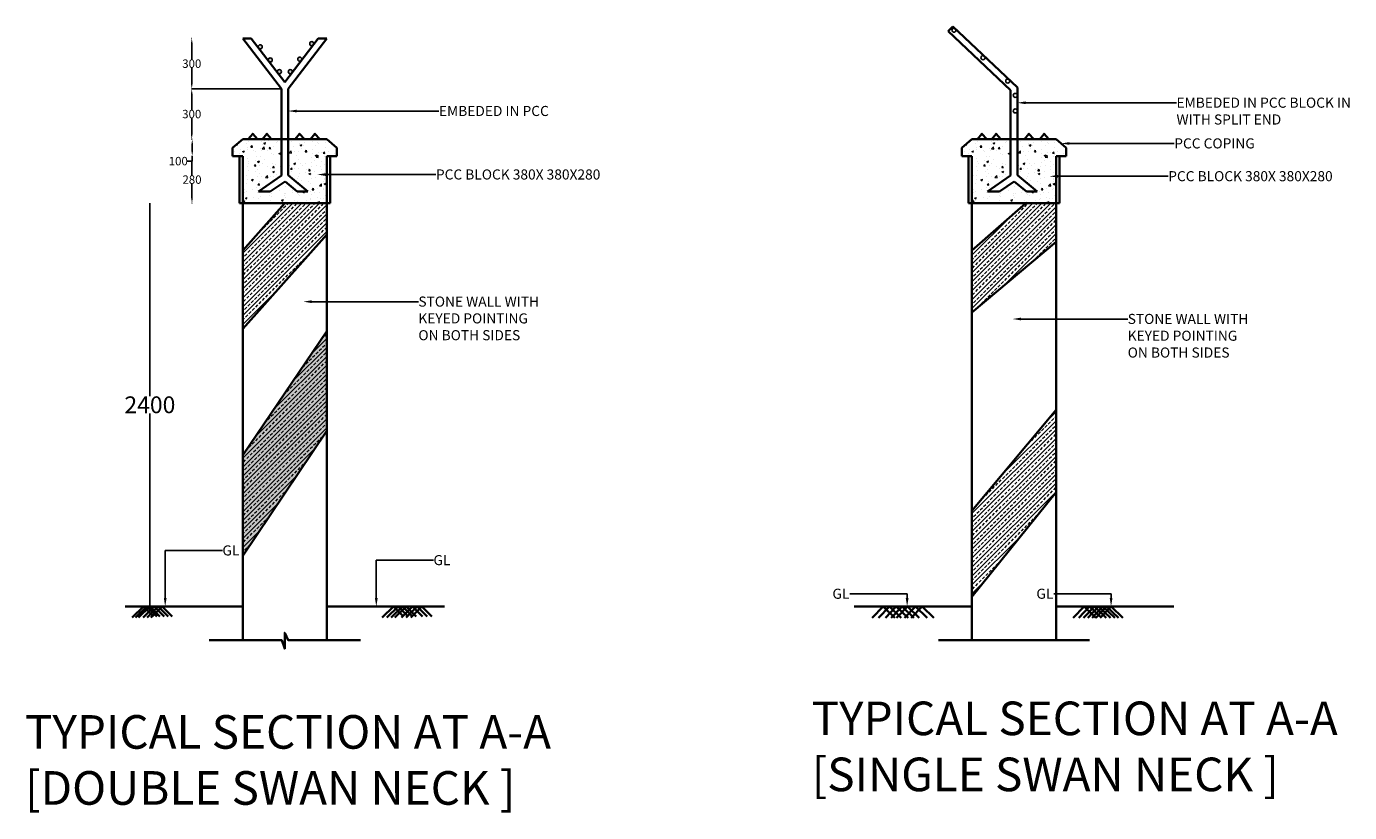
# Model space of a CAD drawing. Units: millimetres. Extents: x 12559 to 31551, y 33148 to 41181.
# Tile 3 of 3: x 23682 to 31551, y 33148 to 37826. Entities that reach past the tile are written whole.
import ezdxf
from ezdxf import colors
from ezdxf.entities.mleader import LeaderData, LeaderLine
from ezdxf.math import Vec2, Vec3

# ---------------------------------------------------------------- set-up
doc = ezdxf.new("R2010")
doc.units = ezdxf.units.MM
doc.header["$MEASUREMENT"] = 0
for name, color, linetype, lineweight in [('A-ANNO-DIMS', 2, 'Continuous', 18), ('A-ANNO-TEXT', 3, 'Continuous', 25), ('A-DETL', 7, 'Continuous', 35), ('A-DETL-PATT', 8, 'Continuous', 13), ('S-REIN', 1, 'Continuous', 25)]:
    doc.layers.add(name, color=color, linetype=linetype, lineweight=lineweight)
doc.styles.get("Standard").update_dxf_attribs({"font": 'arial.ttf'})
doc.dimstyles.get("Standard").update_dxf_attribs({"dimtxt": 100, "dimasz": 0.18, "dimexe": 0.18, "dimexo": 0.0625, "dimgap": 0.09, "dimtad": 0, "dimtih": 1, "dimtoh": 1, "dimdec": 0, "dimzin": 0, "dimdsep": 46, "dimtxsty": 'Standard', "dimcen": 0.09, "dimadec": 0, "dimazin": 0, "dimtfac": 1, "dimtdec": 0, "dimtofl": 0, "dimtmove": 0, "dimatfit": 3, "dimfxl": 1, "dimtolj": 1, "dimtzin": 0, "dimarcsym": 0})

# ---------------------------------------------------------------- blocks, each defined once
blk = doc.blocks.new('*D30')
at = {"layer": 'A-ANNO-DIMS', "color": 0, "lineweight": -2, "transparency": 16777216}
for p, q in [((24667.4, 37054.2), (24665.9, 37054.2)), ((24666.1, 37024.2), (24666.1, 36939.8)), ((24666.1, 36804.2), (24666.1, 36888.6)), ((24667.4, 36774.2), (24665.9, 36774.2))]:
    blk.add_line(p, q, dxfattribs=at)
at = {"layer": 'A-ANNO-DIMS', "color": 0, "transparency": 16777216}
for points in [[(24661.1, 37024.2), (24671.1, 37024.2), (24666.1, 37054.2)], [(24661.1, 36804.2), (24671.1, 36804.2), (24666.1, 36774.2)]]:
    blk.add_solid(points, dxfattribs=at)
at = {"layer": 'DEFPOINTS', "color": 0, "transparency": 16777216}
for p in [(24667.4, 37054.2), (24666.1, 36774.2), (24667.4, 36774.2)]:
    blk.add_point(p, dxfattribs=at)
at = {"layer": 'A-ANNO-DIMS', "color": 0, "transparency": 16777216, "insert": (24666.1, 36914.2), "char_height": 50, "attachment_point": 5}
blk.add_mtext('\\A1;280', dxfattribs=at)
blk = doc.blocks.new('*D31')
at = {"layer": 'A-ANNO-DIMS', "color": 0, "lineweight": -2, "transparency": 16777216}
for p, q in [((24663.1, 37154.2), (24667.6, 37154.2)), ((24667.4, 37124.2), (24667.4, 37084.2)), ((24667.4, 37024.2), (24637.4, 37024.2)), ((24666.1, 37054.2), (24667.6, 37054.2)), ((24667.4, 37054.2), (24667.4, 37024.2))]:
    blk.add_line(p, q, dxfattribs=at)
at = {"layer": 'A-ANNO-DIMS', "color": 0, "transparency": 16777216}
for points in [[(24662.4, 37124.2), (24672.4, 37124.2), (24667.4, 37154.2)], [(24662.4, 37084.2), (24672.4, 37084.2), (24667.4, 37054.2)]]:
    blk.add_solid(points, dxfattribs=at)
at = {"layer": 'DEFPOINTS', "color": 0, "transparency": 16777216}
for p in [(24663, 37154.2), (24666.1, 37054.2), (24667.4, 37054.2)]:
    blk.add_point(p, dxfattribs=at)
at = {"layer": 'A-ANNO-DIMS', "color": 0, "transparency": 16777216, "insert": (24584.5, 37024.2), "char_height": 50, "attachment_point": 5}
blk.add_mtext('\\A1;100', dxfattribs=at)
blk = doc.blocks.new('*D32')
at = {"layer": 'A-ANNO-DIMS', "color": 0, "lineweight": -2, "transparency": 16777216}
for p, q in [((25197.8, 37454.2), (24664.3, 37454.2)), ((24664.5, 37424.2), (24664.5, 37329.9)), ((24664.5, 37184.2), (24664.5, 37278.6)), ((24663.1, 37154.2), (24664.6, 37154.2))]:
    blk.add_line(p, q, dxfattribs=at)
at = {"layer": 'A-ANNO-DIMS', "color": 0, "transparency": 16777216}
for points in [[(24659.5, 37424.2), (24669.5, 37424.2), (24664.5, 37454.2)], [(24659.5, 37184.2), (24669.5, 37184.2), (24664.5, 37154.2)]]:
    blk.add_solid(points, dxfattribs=at)
at = {"layer": 'DEFPOINTS', "color": 0, "transparency": 16777216}
for p in [(24664.5, 37454.2), (25197.8, 37454.2), (24663, 37154.2)]:
    blk.add_point(p, dxfattribs=at)
at = {"layer": 'A-ANNO-DIMS', "color": 0, "transparency": 16777216, "insert": (24664.5, 37304.2), "char_height": 50, "attachment_point": 5}
blk.add_mtext('\\A1;300', dxfattribs=at)
blk = doc.blocks.new('*D33')
at = {"layer": 'A-ANNO-DIMS', "color": 0, "lineweight": -2, "transparency": 16777216}
for p, q in [((24664.1, 37754.2), (24665, 37754.2)), ((24664.8, 37724.2), (24664.8, 37629.9)), ((24664.8, 37484.2), (24664.8, 37578.6)), ((24664.1, 37454.2), (24665, 37454.2))]:
    blk.add_line(p, q, dxfattribs=at)
at = {"layer": 'A-ANNO-DIMS', "color": 0, "transparency": 16777216}
for points in [[(24659.8, 37724.2), (24669.8, 37724.2), (24664.8, 37754.2)], [(24659.8, 37484.2), (24669.8, 37484.2), (24664.8, 37454.2)]]:
    blk.add_solid(points, dxfattribs=at)
at = {"layer": 'DEFPOINTS', "color": 0, "transparency": 16777216}
for p in [(24664.1, 37754.2), (24664.1, 37454.2), (24664.8, 37454.2)]:
    blk.add_point(p, dxfattribs=at)
at = {"layer": 'A-ANNO-DIMS', "color": 0, "transparency": 16777216, "insert": (24664.8, 37604.2), "char_height": 50, "attachment_point": 5}
blk.add_mtext('\\A1;300', dxfattribs=at)
blk = doc.blocks.new('*D34')
at = {"layer": 'A-ANNO-DIMS', "color": 0, "lineweight": -2, "transparency": 16777216}
for p, q in [((24416.2, 36774.2), (24415.5, 36774.2)), ((24415.7, 36774), (24415.7, 35625.4)), ((24415.7, 34374.4), (24415.7, 35523.1)), ((24416.2, 34374.2), (24415.5, 34374.2))]:
    blk.add_line(p, q, dxfattribs=at)
at = {"layer": 'A-ANNO-DIMS', "color": 0, "transparency": 16777216}
for points in [[(24415.7, 36774), (24415.7, 36774), (24415.7, 36774.2)], [(24415.7, 34374.4), (24415.7, 34374.4), (24415.7, 34374.2)]]:
    blk.add_solid(points, dxfattribs=at)
at = {"layer": 'DEFPOINTS', "color": 0, "transparency": 16777216}
for p in [(24416.3, 36774.2), (24415.7, 34374.2), (24416.3, 34374.2)]:
    blk.add_point(p, dxfattribs=at)
at = {"layer": 'A-ANNO-DIMS', "color": 0, "transparency": 16777216, "insert": (24415.7, 35574.2), "char_height": 100, "attachment_point": 5}
blk.add_mtext('\\A1;2400', dxfattribs=at)

msp = doc.modelspace()

# ---------------------------------------------------------------- hatches: boundary and pattern name
at = {"layer": 'A-DETL-PATT'}
h = msp.add_hatch(color=256, dxfattribs=at)
h.dxf.hatch_style = 1
h.paths.add_polyline_path([(25366.1, 37723.2, 1), (25390.5, 37723.2, 1)])
h.paths.add_polyline_path([(25295, 37630.6, 1), (25319.4, 37630.6, 1)])
h.paths.add_polyline_path([(25238.2, 37556.5, 1), (25262.6, 37556.5, 1)])
h.paths.add_polyline_path([(25173.5, 37556.6, 1), (25197.9, 37556.6, 1)])
h.paths.add_polyline_path([(25119.5, 37626.5, 1), (25143.9, 37626.5, 1)])
h.paths.add_polyline_path([(25059.7, 37704.1, 0.136284), (25061.5, 37697.8), (25063.2, 37695.6, 0.675083), (25084.1, 37704.1, 1)])
h = msp.add_hatch(dxfattribs=at)
h.set_pattern_fill('AR-CONC', color=256, scale=15)
h.set_pattern_definition([(50, (0, 0), (107.58903, -9.41282), [11.25, -123.75]), (355, (0, 0), (-20.8127, 112.82882), [9, -99]), (100.45144, (8.97, -0.78), (86.77633, 103.416), [9.56103, -105.17132]), (46.1842, (0, 30), (160.0862, -24.8279), [16.875, -185.625]), (96.63564, (13.34, 27.93), (140.1993, 146.1178), [14.34155, -157.75706]), (351.18416, (0, 30), (140.1993, 146.1178), [13.5, -148.5]), (21, (15, 22.5), (89.53606, -60.39283), [11.25, -123.75]), (326, (15, 22.5), (36.4973, 108.7725), [9, -99]), (71.45144, (22.46, 17.47), (126.03336, 48.37967), [9.56103, -105.17132]), (37.5, (0, 0), (1.823978, 49.934078), [0, -97.8, 0, -100.5, 0, -99.375]), (7.5, (0, 0), (39.46043, 59.161757), [0, -57.3, 0, -95.55, 0, -37.875]), (327.5, (-33.45, 0), (80.073365, -3.38323), [0, -37.5, 0, -117, 0, -155.25]), (317.5, (-48.45, 0), (87.47793, 15.01575), [0, -48.75, 0, -77.7, 0, -110.25])])
h.paths.add_polyline_path([(25467.8, 37054.2), (25527.8, 37054.2), (25527.8, 37104.2), (25467.8, 37154.2), (25237.8, 37154.2), (25237.8, 36940.5), (25354.9, 36842.6), (25292.6, 36842.6), (25219.3, 36903.9), (25131, 36842.6), (25060.8, 36842.6), (25197.8, 36937.7), (25197.8, 37154.2), (24967.8, 37154.2), (24907.8, 37104.2), (24907.8, 37054.2), (24967.8, 37054.2), (24967.8, 36774.2), (25467.8, 36774.2)])
h = msp.add_hatch(dxfattribs=at)
h.set_pattern_fill('AR-CONC', color=256, scale=15)
h.set_pattern_definition([(50, (4337.23, 0), (107.58903, -9.41282), [11.25, -123.75]), (355, (4337.23, 0), (-20.8127, 112.82882), [9, -99]), (100.45144, (4346.2, -0.78), (86.77633, 103.416), [9.56103, -105.17132]), (46.1842, (4337.23, 30), (160.0862, -24.8279), [16.875, -185.625]), (96.63564, (4350.57, 27.93), (140.1993, 146.1178), [14.34155, -157.75706]), (351.18416, (4337.23, 30), (140.1993, 146.1178), [13.5, -148.5]), (21, (4352.23, 22.5), (89.53606, -60.39283), [11.25, -123.75]), (326, (4352.23, 22.5), (36.4973, 108.7725), [9, -99]), (71.45144, (4359.69, 17.47), (126.03336, 48.37967), [9.56103, -105.17132]), (37.5, (4337.233, 0), (1.823978, 49.934078), [0, -97.8, 0, -100.5, 0, -99.375]), (7.5, (4337.233, 0), (39.46043, 59.161757), [0, -57.3, 0, -95.55, 0, -37.875]), (327.5, (4303.783, 0), (80.073365, -3.38323), [0, -37.5, 0, -117, 0, -155.25]), (317.5, (4288.78, 0), (87.47793, 15.01575), [0, -48.75, 0, -77.7, 0, -110.25])])
h.paths.add_polyline_path([(29805.1, 37054.2), (29865.1, 37054.2), (29865.1, 37104.2), (29805.1, 37154.2), (29575.1, 37154.2), (29575.1, 36940.5), (29692.1, 36842.6), (29629.8, 36842.6), (29556.5, 36903.9), (29468.2, 36842.6), (29398.1, 36842.6), (29535.1, 36937.7), (29535.1, 37154.2), (29305.1, 37154.2), (29245.1, 37104.2), (29245.1, 37054.2), (29305.1, 37054.2), (29305.1, 36774.2), (29805.1, 36774.2)])
h = msp.add_hatch(dxfattribs=at)
h.set_pattern_fill('ANSI33', color=256, scale=150)
h.paths.add_polyline_path([(25467.8, 36587.6), (25467.8, 36774.2), (25217.8, 36774.2), (24967.8, 36493.2), (24967.8, 36027.2)])
h = msp.add_hatch(dxfattribs=at)
h.set_pattern_fill('ANSI33', color=256, scale=150)
h.paths.add_polyline_path([(29805.1, 36544.4), (29805.1, 36774.2), (29626.3, 36774.2), (29305.1, 36492.2), (29305.1, 36123.9)])
h = msp.add_hatch(dxfattribs=at)
h.set_pattern_fill('ANSI33', color=256, scale=60)
h.paths.add_polyline_path([(25467.8, 36011.6), (24967.8, 35274.4), (24967.8, 34675.7), (25467.8, 35418.4)])
h = msp.add_hatch(dxfattribs=at)
h.set_pattern_fill('ANSI33', color=256, scale=150)
h.paths.add_polyline_path([(25467.8, 36011.6), (24967.8, 35274.4), (24967.8, 34675.7), (25467.8, 35418.4)])
h = msp.add_hatch(dxfattribs=at)
h.set_pattern_fill('ANSI33', color=256, scale=150)
h.paths.add_polyline_path([(29805.1, 35054.6), (29805.1, 35543.3), (29305.1, 34943.5), (29305.1, 34432.5)])

# ---------------------------------------------------------------- linework, layer by layer
at = {"layer": 'A-DETL'}
for p, q in [((29164.4, 37796.5), (29191.9, 37825.5)), ((29535.1, 37445.6), (29164.4, 37796.5)), ((29575.1, 37462.8), (29191.9, 37825.5)), ((25197.8, 37454.2), (24967.8, 37754.2)), ((25018.2, 37754.2), (24967.8, 37754.2)), ((25217.8, 37493.9), (25018.2, 37754.2)), ((25217.8, 37493.9), (25417.4, 37754.2)), ((25237.8, 37454.2), (25467.8, 37754.2)), ((25467.8, 37754.2), (25417.4, 37754.2)), ((29575.1, 36940.5), (29575.1, 37462.8)), ((25197.8, 36937.7), (25197.8, 37454.2)), ((25237.8, 36940.5), (25237.8, 37454.2)), ((29535.1, 36937.7), (29535.1, 37445.6)), ((24907.8, 37104.2), (24967.8, 37154.2)), ((25467.8, 37154.2), (24967.8, 37154.2)), ((25467.8, 37154.2), (25527.8, 37104.2)), ((29245.1, 37104.2), (29305.1, 37154.2)), ((29805.1, 37154.2), (29305.1, 37154.2)), ((29805.1, 37154.2), (29865.1, 37104.2)), ((24907.8, 37054.2), (24907.8, 37104.2)), ((25527.8, 37054.2), (25527.8, 37104.2)), ((29245.1, 37054.2), (29245.1, 37104.2)), ((29865.1, 37054.2), (29865.1, 37104.2)), ((24967.8, 37054.2), (24907.8, 37054.2)), ((24947.8, 36774.2), (24947.8, 37054.2)), ((24967.8, 34174.2), (24967.8, 37054.2)), ((25467.8, 34174.2), (25467.8, 37054.2)), ((25527.8, 37054.2), (25467.8, 37054.2)), ((25487.8, 36774.2), (25487.8, 37054.2)), ((29305.1, 37054.2), (29245.1, 37054.2)), ((29285.1, 36774.2), (29285.1, 37054.2)), ((29305.1, 34174.2), (29305.1, 37054.2)), ((29805.1, 34174.2), (29805.1, 37054.2)), ((29865.1, 37054.2), (29805.1, 37054.2)), ((29825.1, 36774.2), (29825.1, 37054.2)), ((25197.8, 36937.7), (25060.8, 36842.6)), ((25237.8, 36940.5), (25354.9, 36842.6)), ((29535.1, 36937.7), (29398.1, 36842.6)), ((29575.1, 36940.5), (29692.1, 36842.6)), ((25060.8, 36842.6), (25131, 36842.6)), ((25219.3, 36903.9), (25131, 36842.6)), ((25219.3, 36903.9), (25292.6, 36842.6)), ((25292.6, 36842.6), (25354.9, 36842.6)), ((29398.1, 36842.6), (29468.2, 36842.6)), ((29556.5, 36903.9), (29468.2, 36842.6)), ((29556.5, 36903.9), (29629.8, 36842.6)), ((29629.8, 36842.6), (29692.1, 36842.6)), ((25487.8, 36774.2), (24947.8, 36774.2)), ((25217.8, 36774.2), (24967.8, 36493.2)), ((29825.1, 36774.2), (29285.1, 36774.2)), ((29626.3, 36774.2), (29305.1, 36492.2)), ((25467.8, 36587.6), (24967.8, 36027.2)), ((29305.1, 36123.9), (29805.1, 36544.4)), ((24967.8, 35274.4), (25467.8, 36011.6)), ((29305.1, 34943.5), (29805.1, 35543.3)), ((24967.8, 34675.7), (25467.8, 35418.4)), ((29305.1, 34432.5), (29805.1, 35054.6)), ((24767.8, 34374.2), (24267.8, 34374.2)), ((24967.8, 34374.2), (24767.8, 34374.2)), ((25467.8, 34374.2), (25667.8, 34374.2)), ((25667.8, 34374.2), (25467.8, 34374.2)), ((25667.8, 34374.2), (26167.8, 34374.2)), ((29105.1, 34374.2), (28605.1, 34374.2)), ((29305.1, 34374.2), (29105.1, 34374.2)), ((29805.1, 34374.2), (29805.1, 34374.2)), ((29805.1, 34374.2), (30005.1, 34374.2)), ((30005.1, 34374.2), (30505.1, 34374.2)), ((24967.8, 34174.2), (24767.8, 34174.2)), ((25199.5, 34174.2), (24967.8, 34174.2)), ((25667.8, 34174.2), (25237.8, 34174.2)), ((29805.1, 34174.2), (29105.1, 34174.2)), ((29805.1, 34174.2), (30005.1, 34174.2))]:
    msp.add_line(p, q, dxfattribs=at)
for points in [[(25001, 37154.2), (25027.4, 37186.7), (25055.8, 37154.2)], [(25085, 37154.2), (25111.5, 37186.7), (25139.9, 37154.2)], [(25280, 37154.2), (25306.4, 37186.7), (25334.8, 37154.2)], [(25370.8, 37154.2), (25397.3, 37186.7), (25425.7, 37154.2)], [(29338.2, 37154.2), (29364.7, 37186.7), (29393.1, 37154.2)], [(29422.3, 37154.2), (29448.7, 37186.7), (29477.1, 37154.2)], [(29617.2, 37154.2), (29643.7, 37186.7), (29672.1, 37154.2)], [(29708, 37154.2), (29734.5, 37186.7), (29762.9, 37154.2)], [(24310.6, 34308.2), (24376.9, 34374.2), (24436.4, 34314.5)], [(24330.3, 34308.2), (24396.6, 34374.2), (24456.1, 34314.5)], [(24348.7, 34308.2), (24415.1, 34374.2), (24474.5, 34314.5)], [(24374.8, 34308.2), (24441.1, 34374.2), (24500.6, 34314.5)], [(24398.7, 34308.2), (24465, 34374.2), (24524.5, 34314.5)], [(24422.1, 34308.2), (24488.4, 34374.2), (24547.9, 34314.5)], [(25797.5, 34308.2), (25863.8, 34374.2), (25923.3, 34314.5)], [(25825.4, 34308.2), (25891.7, 34374.2), (25951.2, 34314.5)], [(25851.5, 34308.2), (25917.8, 34374.2), (25977.3, 34314.5)], [(25873.4, 34308.2), (25939.8, 34374.2), (25999.2, 34314.5)], [(25911.8, 34308.2), (25978.2, 34374.2), (26037.6, 34314.5)], [(25939.8, 34308.2), (26006.1, 34374.2), (26065.6, 34314.5)], [(25966.8, 34308.2), (26033.2, 34374.2), (26092.6, 34314.5)], [(28711.8, 34306.9), (28776.6, 34374.2), (28846.7, 34306.8)], [(28749.5, 34306.9), (28814.2, 34374.2), (28884.4, 34306.8)], [(28790.3, 34306.9), (28855.1, 34374.2), (28925.2, 34306.8)], [(28825, 34306.9), (28889.8, 34374.2), (28959.9, 34306.8)], [(28856.2, 34306.9), (28920.9, 34374.2), (28991.1, 34306.8)], [(28904.3, 34306.9), (28969.1, 34374.2), (29039.2, 34306.8)], [(28943.9, 34306.9), (29008.7, 34374.2), (29078.8, 34306.8)], [(29907.2, 34306.9), (29972, 34374.2), (30042.1, 34306.8)], [(29940.3, 34306.9), (30005.1, 34374.2), (30075.2, 34306.8)], [(29968.8, 34306.9), (30033.6, 34374.2), (30103.7, 34306.8)], [(29993.7, 34306.9), (30058.5, 34374.2), (30128.7, 34306.8)], [(30019.6, 34306.9), (30084.4, 34374.2), (30154.5, 34306.8)], [(30041, 34306.9), (30105.8, 34374.2), (30175.9, 34306.8)], [(30067.8, 34306.9), (30132.6, 34374.2), (30202.7, 34306.8)], [(24967.6, 34174.2), (25199.5, 34174.2), (25217.7, 34123.1), (25217.9, 34217.6), (25237.8, 34174.2), (25468, 34174.2)]]:
    msp.add_lwpolyline(points, dxfattribs=at)
at = {"layer": 'S-REIN'}
for centre, radius in [((29198, 37803.2), 12), ((25071.9, 37704.1), 12.2), ((25378.3, 37723.2), 12.2), ((25131.7, 37626.5), 12.2), ((25307.2, 37630.6), 12.2), ((29370.8, 37639.7), 12), ((25185.7, 37556.6), 12.2), ((25250.4, 37556.5), 12.2), ((29517.6, 37500.7), 12), ((29563, 37415.5), 12), ((29563, 37322.9), 12)]:
    msp.add_circle(centre, radius, dxfattribs=at)

# ---------------------------------------------------------------- texts
at = {"layer": 'A-ANNO-TEXT', "char_height": 200, "attachment_point": 1}
for s, insert in [('TYPICAL SECTION AT A-A\\P[SINGLE SWAN NECK ]', (28352.1, 33808.5)), ('TYPICAL SECTION AT A-A [DOUBLE SWAN NECK ]', (23673.1, 33727.8))]:
    msp.add_mtext_dynamic_manual_height_columns(s, width=3493.58, gutter_width=1, heights=[0], dxfattribs=dict(at, insert=insert))

# ---------------------------------------------------------------- dimensions: what is measured, and where the dimension line sits
at = {"layer": 'A-ANNO-DIMS'}
for base, p1, p2, override, picture, middle in [((24664.8, 37454.2), (24664.1, 37754.2), (24664.1, 37454.2), {"dimtxt": 50, "dimasz": 30, "dimclrd": 0, "dimclre": 0, "dimclrt": 0}, '*D33', (24664.8, 37604.2)), ((24664.5, 37454.2), (24663, 37154.2), (25197.8, 37454.2), {"dimtxt": 50, "dimasz": 30, "dimclrd": 0, "dimclre": 0, "dimclrt": 0}, '*D32', (24664.5, 37304.2)), ((24667.4, 37054.2), (24663, 37154.2), (24666.1, 37054.2), {"dimtxt": 50, "dimasz": 30, "dimclrd": 0, "dimclre": 0, "dimclrt": 0}, '*D31', (24584.5, 37024.2)), ((24666.1, 36774.2), (24667.4, 37054.2), (24667.4, 36774.2), {"dimtxt": 50, "dimasz": 30, "dimclrd": 0, "dimclre": 0, "dimclrt": 0}, '*D30', (24666.1, 36914.2)), ((24415.7, 34374.2), (24416.3, 36774.2), (24416.3, 34374.2), {"dimclrd": 0, "dimclre": 0, "dimclrt": 0}, '*D34', (24415.7, 35574.2))]:
    dim = msp.add_linear_dim(base=base, p1=p1, p2=p2, angle=90, dimstyle='Standard', override=override, dxfattribs=at)
    dim.commit()
    dim.dimension.update_dxf_attribs({"geometry": picture, "text_midpoint": middle})

# ---------------------------------------------------------------- leaders
at = {"layer": 'A-ANNO-TEXT'}
ml = msp.add_multileader_mtext('Standard', dxfattribs=at)
ml.set_content('EMBEDED IN PCC BLOCK IN\\PWITH SPLIT END', color=256)
ml.set_leader_properties()
ml.build(insert=Vec2(0, 0))
ml.multileader.update_dxf_attribs({"dogleg_length": 339.9, "arrow_head_size": 50})
ctx = ml.context
ctx.base_point, ctx.char_height, ctx.arrow_head_size, ctx.landing_gap_size, ctx.plane_origin = Vec3(30521.4, 37371.4), 60, 50, 0.09, Vec3(29575.1, 37371.4)
notes = []
notes.append((ctx, [(0, (1, 1, 0), (30181.5, 37371.4), (1, 0), 339.9, [(0, [(29575.1, 37371.4)], 0, [])])]))
ctx.mtext.insert, ctx.mtext.flow_direction = Vec3(30521.5, 37401.9), 5
ml = msp.add_multileader_mtext('Standard', dxfattribs=at)
ml.set_content('EMBEDED IN PCC ', color=256)
ml.set_leader_properties()
ml.build(insert=Vec2(0, 0))
ml.multileader.update_dxf_attribs({"dogleg_length": 339.9, "arrow_head_size": 50})
ctx = ml.context
ctx.base_point, ctx.char_height, ctx.arrow_head_size, ctx.landing_gap_size, ctx.plane_origin = Vec3(26134.7, 37322.1), 60, 50, 0.09, Vec3(25237.8, 37322.1)
notes.append((ctx, [(0, (1, 1, 0), (25794.8, 37322.1), (1, 0), 339.9, [(0, [(25237.8, 37322.1)], 0, [])])]))
ctx.mtext.insert, ctx.mtext.flow_direction = Vec3(26134.8, 37352.6), 5
ml = msp.add_multileader_mtext('Standard', dxfattribs=at)
ml.set_content('PCC COPING ', color=256)
ml.set_leader_properties()
ml.build(insert=Vec2(0, 0))
ml.multileader.update_dxf_attribs({"dogleg_length": 339.9, "arrow_head_size": 50})
ctx = ml.context
ctx.base_point, ctx.char_height, ctx.arrow_head_size, ctx.landing_gap_size, ctx.plane_origin = Vec3(30508.4, 37129.2), 60, 50, 0.09, Vec3(29835.1, 37129.2)
notes.append((ctx, [(0, (1, 1, 0), (30168.4, 37129.2), (1, 0), 339.9, [(0, [(29835.1, 37129.2)], 0, [])])]))
ctx.mtext.insert, ctx.mtext.flow_direction = Vec3(30508.4, 37159.7), 5
ml = msp.add_multileader_mtext('Standard', dxfattribs=at)
ml.set_content('PCC BLOCK 380X 380X280', color=256)
ml.set_leader_properties()
ml.build(insert=Vec2(0, 0))
ml.multileader.update_dxf_attribs({"dogleg_length": 339.9, "arrow_head_size": 50})
ctx = ml.context
ctx.base_point, ctx.char_height, ctx.arrow_head_size, ctx.landing_gap_size, ctx.plane_origin = Vec3(26116.8, 36944.3), 60, 50, 0.09, Vec3(25411.1, 36944.3)
notes.append((ctx, [(0, (1, 1, 0), (25776.9, 36944.3), (1, 0), 339.9, [(0, [(25411.1, 36944.3)], 0, [])])]))
ctx.mtext.insert, ctx.mtext.flow_direction = Vec3(26116.9, 36974.8), 5
ml = msp.add_multileader_mtext('Standard', dxfattribs=at)
ml.set_content('PCC BLOCK 380X 380X280', color=256)
ml.set_leader_properties()
ml.build(insert=Vec2(0, 0))
ml.multileader.update_dxf_attribs({"dogleg_length": 339.9, "arrow_head_size": 50})
ctx = ml.context
ctx.base_point, ctx.char_height, ctx.arrow_head_size, ctx.landing_gap_size, ctx.plane_origin = Vec3(30472.3, 36934.1), 60, 50, 0.09, Vec3(29766.6, 36934.1)
notes.append((ctx, [(0, (1, 1, 0), (30132.3, 36934.1), (1, 0), 339.9, [(0, [(29766.6, 36934.1)], 0, [])])]))
ctx.mtext.insert, ctx.mtext.flow_direction = Vec3(30472.4, 36964.6), 5
ml = msp.add_multileader_mtext('Standard', dxfattribs=at)
ml.set_content('STONE WALL WITH\\PKEYED POINTING\\PON BOTH SIDES', color=256)
ml.set_leader_properties()
ml.build(insert=Vec2(0, 0))
ml.multileader.update_dxf_attribs({"dogleg_length": 339.9, "arrow_head_size": 50})
ctx = ml.context
ctx.base_point, ctx.char_height, ctx.arrow_head_size, ctx.landing_gap_size, ctx.plane_origin = Vec3(26012.4, 36187.9), 60, 50, 0.09, Vec3(25327.6, 36187.9)
notes.append((ctx, [(0, (1, 1, 0), (25672.5, 36187.9), (1, 0), 339.9, [(0, [(25327.6, 36187.9)], 0, [])])]))
ctx.mtext.insert, ctx.mtext.flow_direction = Vec3(26012.5, 36218.4), 5
ml = msp.add_multileader_mtext('Standard', dxfattribs=at)
ml.set_content('STONE WALL WITH\\PKEYED POINTING\\PON BOTH SIDES', color=256)
ml.set_leader_properties()
ml.build(insert=Vec2(0, 0))
ml.multileader.update_dxf_attribs({"dogleg_length": 339.9, "arrow_head_size": 50})
ctx = ml.context
ctx.base_point, ctx.char_height, ctx.arrow_head_size, ctx.landing_gap_size, ctx.plane_origin = Vec3(30231.3, 36084.7), 60, 50, 0.09, Vec3(29546.4, 36084.7)
notes.append((ctx, [(0, (1, 1, 0), (29891.3, 36084.7), (1, 0), 339.9, [(0, [(29546.4, 36084.7)], 0, [])])]))
ctx.mtext.insert, ctx.mtext.flow_direction = Vec3(30231.3, 36115.2), 5
ml = msp.add_multileader_mtext('Standard', dxfattribs=at)
ml.set_content('GL ', color=256)
ml.set_leader_properties()
ml.build(insert=Vec2(0, 0))
ml.multileader.update_dxf_attribs({"dogleg_length": 339.9, "arrow_head_size": 50})
ctx = ml.context
ctx.base_point, ctx.char_height, ctx.arrow_head_size, ctx.landing_gap_size, ctx.plane_origin = Vec3(24846.8, 34707.2), 60, 50, 0.09, Vec3(24506.8, 34374.2)
notes.append((ctx, [(0, (1, 1, 0), (24506.8, 34707.2), (1, 0), 339.9, [(0, [(24506.8, 34374.2)], 0, [])])]))
ctx.mtext.insert, ctx.mtext.flow_direction = Vec3(24846.9, 34737.7), 5
ml = msp.add_multileader_mtext('Standard', dxfattribs=at)
ml.set_content('GL ', color=256)
ml.set_leader_properties()
ml.build(insert=Vec2(0, 0))
ml.multileader.update_dxf_attribs({"dogleg_length": 339.9, "arrow_head_size": 50})
ctx = ml.context
ctx.base_point, ctx.char_height, ctx.arrow_head_size, ctx.landing_gap_size, ctx.plane_origin = Vec3(26102.3, 34649.5), 60, 50, 0.09, Vec3(25762.3, 34374.2)
notes.append((ctx, [(0, (1, 1, 0), (25762.3, 34649.5), (1, 0), 339.9, [(0, [(25762.3, 34374.2)], 0, [])])]))
ctx.mtext.insert, ctx.mtext.flow_direction = Vec3(26102.4, 34680), 5
ml = msp.add_multileader_mtext('Standard', dxfattribs=at)
ml.set_content('GL', color=256)
ml.set_leader_properties()
ml.build(insert=Vec2(0, 0))
ml.multileader.update_dxf_attribs({"dogleg_length": 339.9, "arrow_head_size": 50})
ctx = ml.context
ctx.base_point, ctx.char_height, ctx.arrow_head_size, ctx.landing_gap_size, ctx.plane_origin = Vec3(28475, 34449.5), 60, 50, 0.09, Vec3(28919.5, 34374.2)
notes.append((ctx, [(0, (1, 1, 0), (28919.5, 34449.5), (-1, 0), 339.9, [(0, [(28919.5, 34374.2)], 0, [])])]))
ctx.mtext.insert, ctx.mtext.flow_direction = Vec3(28475.1, 34480), 5
ml = msp.add_multileader_mtext('Standard', dxfattribs=at)
ml.set_content('GL', color=256)
ml.set_leader_properties()
ml.build(insert=Vec2(0, 0))
ml.multileader.update_dxf_attribs({"dogleg_length": 339.9, "arrow_head_size": 50})
ctx = ml.context
ctx.base_point, ctx.char_height, ctx.arrow_head_size, ctx.landing_gap_size, ctx.plane_origin = Vec3(29688.1, 34449.5), 60, 50, 0.09, Vec3(30132.6, 34374.2)
notes.append((ctx, [(0, (1, 1, 0), (30132.6, 34449.5), (-1, 0), 339.9, [(0, [(30132.6, 34374.2)], 0, [])])]))
ctx.mtext.insert, ctx.mtext.flow_direction = Vec3(29688.2, 34480), 5
for ctx, leaders in notes:
    for number, flags, end, landing, length, lines in leaders:
        leader = LeaderData()
        leader.index, (leader.has_last_leader_line, leader.has_dogleg_vector, leader.attachment_direction) = number, flags
        leader.last_leader_point, leader.dogleg_vector, leader.dogleg_length = Vec3(end), Vec3(landing), length
        for number, points, colour, breaks in lines:
            line = LeaderLine()
            line.index, line.vertices, line.color, line.breaks = number, Vec3.list(points), colors.encode_raw_color(colour), breaks
            leader.lines.append(line)
        ctx.leaders.append(leader)

doc.saveas('drawing.dxf')
